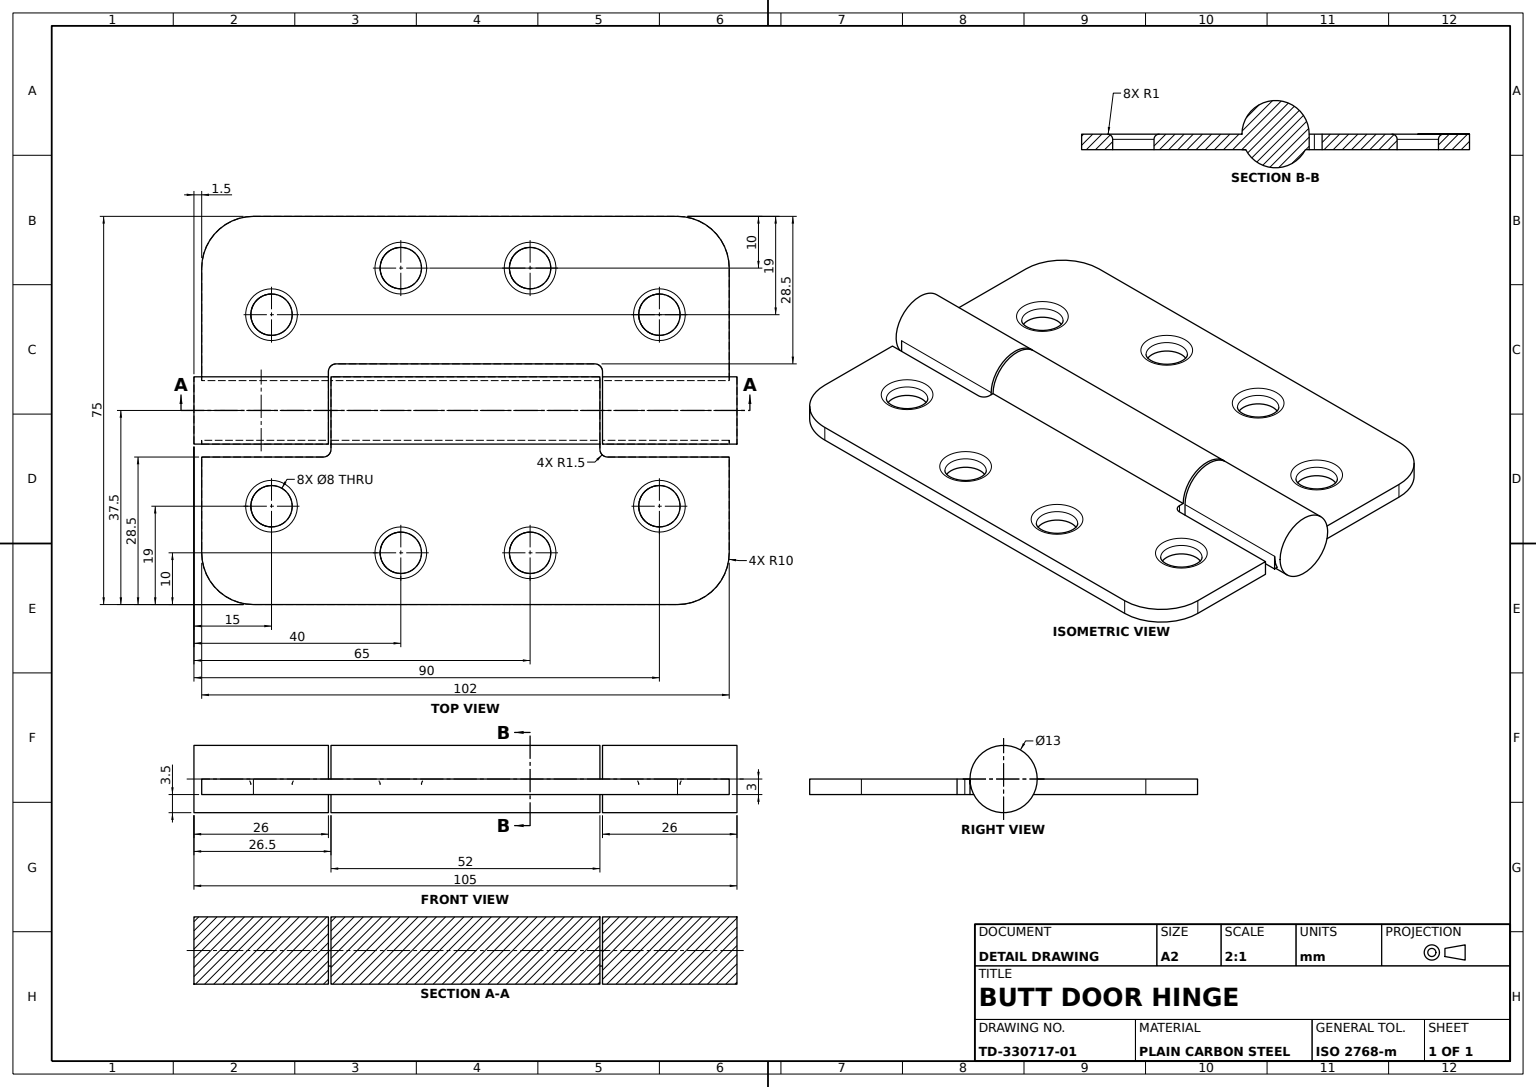
from build123d import *

# Parameters (mm, degrees)
HINGE_LEAVES_3MM_DEPTH        = 3
HINGE_LEAVES_3MM_2_DEPTH      = 3
SCREW_HOLES_PROFILE_R         = 4
SCREW_HOLES_8X_8_DEPTH        = 3
SCREW_HOLE_EDGE_FILLET_R1_A_R = 1
SCREW_HOLE_EDGE_FILLET_R1_B_R = 1
END_KNUCKLE_1_PROFILE_W       = 26
END_KNUCKLE_1_PROFILE_H       = 6.5
CENTRE_KNUCKLE_PROFILE_W      = 52
CENTRE_KNUCKLE_PROFILE_H      = 6.5
END_KNUCKLE_2_PROFILE_W       = 26
END_KNUCKLE_2_PROFILE_H       = 6.5


with BuildPart() as part:
    # Hinge Leaves Profile → Hinge Leaves 3mm (new body)
    with BuildSketch(Plane(origin=(0, 0, 0), x_dir=(1, 0, 0), z_dir=(0, 1, 0))):
        with BuildLine():
            Line((0, 0), (0, -6.5))
            Line((0, -6.5), (24.5, -6.5))
            Line((24.5, -6.5), (24.5, 7.5))
            ThreePointArc((24.5, 7.5), (24.939339828, 8.560660172), (26, 9))
            Line((26, 9), (76, 9))
            ThreePointArc((76, 9), (77.060660172, 8.560660172), (77.5, 7.5))
            Line((77.5, 7.5), (77.5, -6.5))
            Line((77.5, -6.5), (102, -6.5))
            Line((102, -6.5), (102, 27.5))
            ThreePointArc((102, 27.5), (99.071067812, 34.571067812), (92, 37.5))
            Line((92, 37.5), (10, 37.5))
            ThreePointArc((10, 37.5), (2.928932188, 34.571067812), (0, 27.5))
            Line((0, 27.5), (0, 0))
        make_face()
    extrude(amount=-HINGE_LEAVES_3MM_DEPTH)


with BuildPart() as body_2:
    # Hinge Leaves Profile → Hinge Leaves 3mm 2 (new body)
    with BuildSketch(Plane(origin=(0, 0, 0), x_dir=(1, 0, 0), z_dir=(0, 1, 0))):
        with BuildLine():
            Line((0, -9), (23.5, -9))
            ThreePointArc((23.5, -9), (24.560660172, -8.560660172), (25, -7.5))
            Line((25, -7.5), (25, 6.5))
            Line((25, 6.5), (77, 6.5))
            Line((77, 6.5), (77, -7.5))
            ThreePointArc((77, -7.5), (77.439339828, -8.560660172), (78.5, -9))
            Line((78.5, -9), (102, -9))
            Line((102, -9), (102, -27.5))
            ThreePointArc((102, -27.5), (99.071067812, -34.571067812), (92, -37.5))
            Line((92, -37.5), (10, -37.5))
            ThreePointArc((10, -37.5), (2.928932188, -34.571067812), (0, -27.5))
            Line((0, -27.5), (0, -9))
        make_face()
    extrude(amount=-HINGE_LEAVES_3MM_2_DEPTH)


with BuildPart() as screw_holes_8x_8_tool:
    # Screw Holes Profile → Screw Holes 8xØ8 (new body)
    with BuildSketch(Plane(origin=(0, 0, 0), x_dir=(1, 0, 0), z_dir=(0, 1, 0))):
        with Locations(Location((13.5, 18.5, 0), (0, 0, 270))):
            Circle(SCREW_HOLES_PROFILE_R)
        with Locations(Location((38.5, 27.5, 0), (0, 0, 270))):
            Circle(SCREW_HOLES_PROFILE_R)
        with Locations(Location((63.5, 27.5, 0), (0, 0, 270))):
            Circle(SCREW_HOLES_PROFILE_R)
        with Locations(Location((88.5, 18.5, 0), (0, 0, 270))):
            Circle(SCREW_HOLES_PROFILE_R)
        with Locations(Location((13.5, -18.5, 0), (0, 0, 270))):
            Circle(SCREW_HOLES_PROFILE_R)
        with Locations(Location((38.5, -27.5, 0), (0, 0, 270))):
            Circle(SCREW_HOLES_PROFILE_R)
        with Locations(Location((63.5, -27.5, 0), (0, 0, 270))):
            Circle(SCREW_HOLES_PROFILE_R)
        with Locations(Location((88.5, -18.5, 0), (0, 0, 270))):
            Circle(SCREW_HOLES_PROFILE_R)
    extrude(amount=-SCREW_HOLES_8X_8_DEPTH)


with BuildPart() as part_1:
    add(part.part)

    # Screw Holes 8xØ8: cut by screw_holes_8x_8_tool
    add(screw_holes_8x_8_tool.part, mode=Mode.SUBTRACT)

    # Screw Hole Edge Fillet R1 A
    screw_hole_edge_fillet_r1_a_edges = [part_1.edges().sort_by_distance(p)[0] for p in [
        (13.5, 0, -22.5),
        (38.5, 0, -31.5),
        (63.5, 0, -31.5),
        (88.5, 0, -22.5),
    ]]
    fillet(screw_hole_edge_fillet_r1_a_edges, radius=SCREW_HOLE_EDGE_FILLET_R1_A_R)

    # End Knuckle 1 Profile → End Knuckle 1 Ø13x26 (revolve)
    with BuildSketch(Plane.XY):
        with Locations((11.5, 3.25)):
            Rectangle(END_KNUCKLE_1_PROFILE_W, END_KNUCKLE_1_PROFILE_H)
    revolve(axis=Axis((24.5, 0, 0), (-1, 0, 0)))

    # End Knuckle 2 Profile → End Knuckle 2 Ø13x26 (revolve)
    with BuildSketch(Plane.XY, mode=Mode.PRIVATE) as end_knuckle_2_13x26_sk:
        with Locations((90.5, 3.25)):
            Rectangle(END_KNUCKLE_2_PROFILE_W, END_KNUCKLE_2_PROFILE_H)
    revolve(end_knuckle_2_13x26_sk.sketch.rotate(Axis((77.5, 0, 0), (1, 0, 0)), 90), axis=Axis((77.5, 0, 0), (1, 0, 0)))


with BuildPart() as body_2_1:
    add(body_2.part)

    # Screw Holes 8xØ8: cut by screw_holes_8x_8_tool
    add(screw_holes_8x_8_tool.part, mode=Mode.SUBTRACT)

    # Screw Hole Edge Fillet R1 B
    screw_hole_edge_fillet_r1_b_edges = [body_2_1.edges().sort_by_distance(p)[0] for p in [
        (13.5, 0, 14.5),
        (38.5, 0, 23.5),
        (63.5, 0, 23.5),
        (88.5, 0, 14.5),
    ]]
    fillet(screw_hole_edge_fillet_r1_b_edges, radius=SCREW_HOLE_EDGE_FILLET_R1_B_R)

    # Centre Knuckle Profile → Centre Knuckle Ø13x52 (revolve)
    with BuildSketch(Plane.XY):
        with Locations((51, 3.25)):
            Rectangle(CENTRE_KNUCKLE_PROFILE_W, CENTRE_KNUCKLE_PROFILE_H)
    revolve(axis=Axis((25, 0, 0), (1, 0, 0)))


solid = Compound([part_1.part, body_2_1.part])
